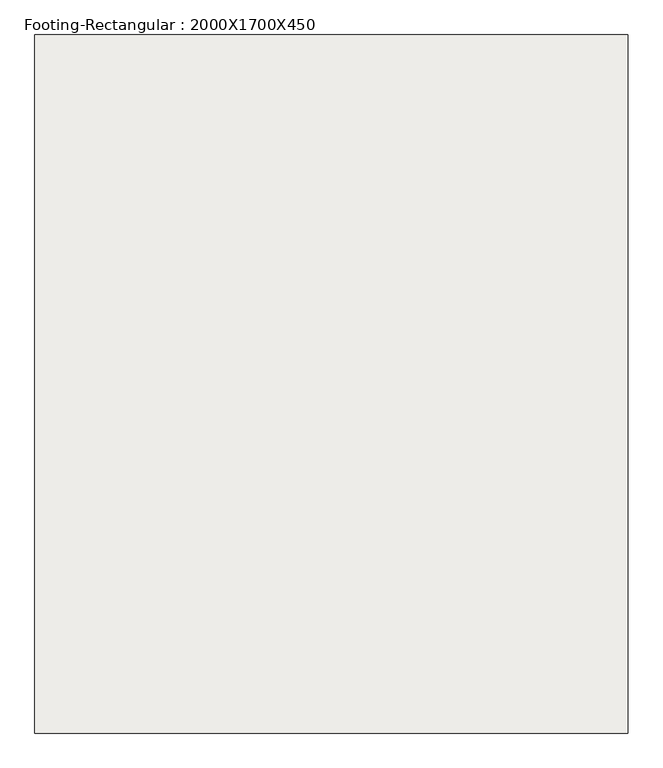
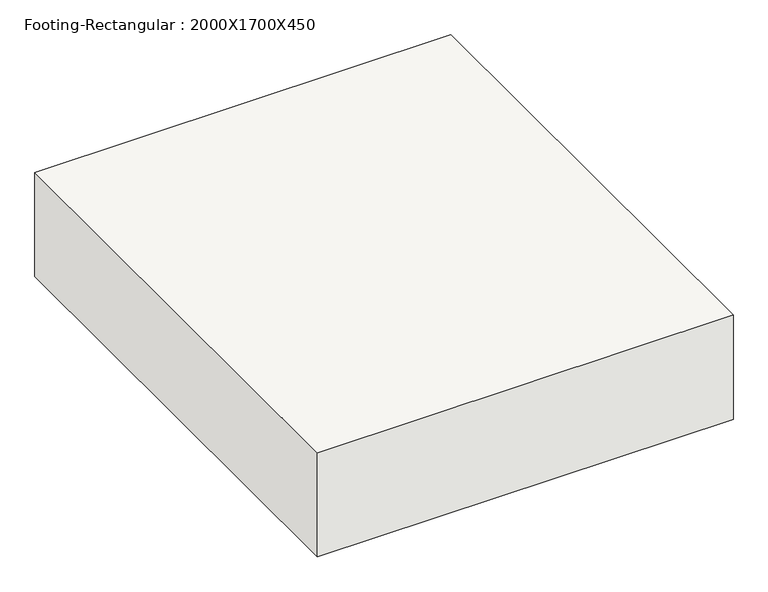
"""IFC4 building model written with IfcOpenShell, lengths in millimetres: slab geometry, Footing-Rectangular : 2000X1700X450."""

from ifc_helpers import new_model, si_unit, frame, origin, place, context, project, spatial, polyline, outline, extrude, source, transform, mapped, element, save


def footing_rectangular_2000x1700x450_8886efa8(model_context):
    return source(origin(), model_context, "Body", "SweptSolid", [
        extrude(outline(polyline([(850.0, 1000.0), (850.0, -1000.0), (-850.0, -1000.0), (-850.0, 1000.0), (850.0, 1000.0)])), frame((0.0, 0.0, -450.0), z_axis=(0.0, 0.0, 1.0), x_axis=(1.0, 0.0, 0.0)), (0.0, 0.0, 1.0), 450.0),
    ])


if __name__ == "__main__":
    model = new_model("IFC4")
    model_context = context("Model", 3, world=origin())
    ifc_project = project(units=[si_unit("LENGTHUNIT", "METRE", prefix="MILLI")], contexts=[model_context])
    site = spatial("IfcSite", under=ifc_project)
    building = spatial("IfcBuilding", under=site)
    placement = place(None, origin())
    footing_rectangular_2000x1700x450_shape = footing_rectangular_2000x1700x450_8886efa8(model_context)
    element("IfcSlab", 1, ObjectType="Footing-Rectangular : 2000X1700X450", at=placement, inside=building, context=model_context, shape_type="MappedRepresentation", body=[
        mapped(footing_rectangular_2000x1700x450_shape, transform((0.0, 0.0, 0.0), x_axis=(1.0, 0.0, 0.0), y_axis=(0.0, 1.0, 0.0), z_axis=(0.0, 0.0, 1.0))),
    ])
    save(model, "model.ifc")

# Revit data of these elements
# Type "Footing-Rectangular : 2000X1700X450"
#   Width = 5' - 6.92913"
#   Length = 6' - 6.74016"
#   Foundation Thickness = 1' - 5.71654"
#   Structural Material [instance default] = Concrete - Cast-in-Place Concrete
#   Assembly Code = ""
# Element 1 (IfcSlab, "Footing-Rectangular : 2000X1700X450")
#   Materials on its faces: "Concrete - Cast-in-Place Concrete"
# Materials
#   "Concrete - Cast-in-Place Concrete": class "Concrete", colour RGB 192 192 192, transparency 0, Cost = 0
